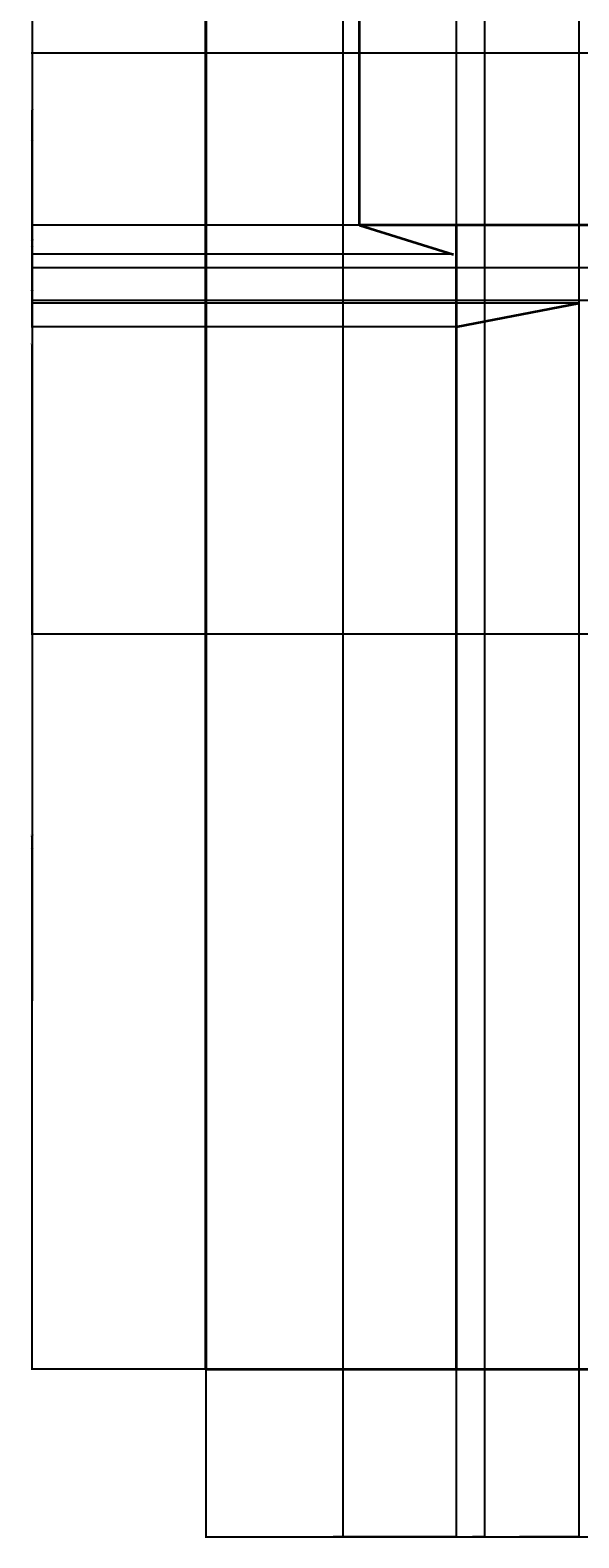
# Model space of a CAD drawing. Units: feet. Extents: x 4092 to 5585, y 725 to 1390.
# Tile 2 of 7: x 4921 to 5022, y 725 to 1001. Entities that reach past the tile are written whole.
import ezdxf

# ---------------------------------------------------------------- set-up
doc = ezdxf.new("R2010")
doc.units = ezdxf.units.FT
doc.layers.add('A-ANNO-DIMS', color=2, linetype='Continuous', lineweight=18)
doc.layers.add('A-ELEV', color=7, linetype='Continuous', lineweight=35)
doc.styles.get("Standard").update_dxf_attribs({"font": 'arial.ttf'})
doc.dimstyles.get("Standard").update_dxf_attribs({"dimtxt": 0.18, "dimasz": 0.18, "dimexe": 0.18, "dimexo": 0.0625, "dimgap": 0.09, "dimtad": 0, "dimtih": 1, "dimtoh": 1, "dimdec": 1, "dimzin": 0, "dimdsep": 46, "dimlunit": 3, "dimtxsty": 'Standard', "dimcen": 0.09, "dimadec": 0, "dimazin": 0, "dimtfac": 1, "dimtdec": 1, "dimtofl": 0, "dimtmove": 0, "dimatfit": 3, "dimfxl": 1, "dimtolj": 1, "dimtzin": 0, "dimarcsym": 0})

# ---------------------------------------------------------------- blocks, each defined once
blk = doc.blocks.new('*D4')
at = {"layer": 'A-ANNO-DIMS', "color": 0, "lineweight": -2, "transparency": 16777216}
for p, q in [((4953.29, 755.89), (4953.29, 725.07)), ((5553.29, 755.89), (5553.29, 725.07)), ((4953.47, 725.25), (5253, 725.25)), ((5553.11, 725.25), (5253.58, 725.25))]:
    blk.add_line(p, q, dxfattribs=at)
at = {"layer": 'A-ANNO-DIMS', "color": 0, "transparency": 16777216}
for points in [[(4953.47, 725.28), (4953.47, 725.22), (4953.29, 725.25)], [(5553.11, 725.28), (5553.11, 725.22), (5553.29, 725.25)]]:
    blk.add_solid(points, dxfattribs=at)
at = {"layer": 'Defpoints', "color": 0, "transparency": 16777216}
for p in [(4953.29, 755.95), (5553.29, 755.95), (5553.29, 725.25)]:
    blk.add_point(p, dxfattribs=at)
at = {"layer": 'A-ANNO-DIMS', "color": 0, "transparency": 16777216, "insert": (5253.29, 725.25), "char_height": 0.18, "attachment_point": 5}
blk.add_mtext('\\A1;600', dxfattribs=at)
blk = doc.blocks.new('*D17')
at = {"layer": 'A-ANNO-DIMS', "color": 0, "lineweight": -2, "transparency": 16777216}
for p, q in [((5021.54, 951.2), (4921.27, 951.2)), ((4921.45, 951.02), (4921.45, 853.76)), ((4921.45, 756.13), (4921.45, 853.39)), ((5285.73, 755.95), (4921.27, 755.95))]:
    blk.add_line(p, q, dxfattribs=at)
at = {"layer": 'A-ANNO-DIMS', "color": 0, "transparency": 16777216}
for points in [[(4921.42, 951.02), (4921.48, 951.02), (4921.45, 951.2)], [(4921.42, 756.13), (4921.48, 756.13), (4921.45, 755.95)]]:
    blk.add_solid(points, dxfattribs=at)
at = {"layer": 'Defpoints', "color": 0, "transparency": 16777216}
for p in [(4921.45, 951.2), (5021.61, 951.2), (5285.79, 755.95)]:
    blk.add_point(p, dxfattribs=at)
at = {"layer": 'A-ANNO-DIMS', "color": 0, "transparency": 16777216, "insert": (4921.45, 853.58), "char_height": 0.18, "attachment_point": 5}
blk.add_mtext('\\A1;195.25', dxfattribs=at)
blk = doc.blocks.new('*D18')
at = {"layer": 'A-ANNO-DIMS', "color": 0, "lineweight": -2, "transparency": 16777216}
for p, q in [((4978.29, 1010.79), (4921.27, 1010.79)), ((4921.45, 1010.61), (4921.45, 981.18)), ((4921.45, 951.38), (4921.45, 980.81)), ((5021.54, 951.2), (4921.27, 951.2))]:
    blk.add_line(p, q, dxfattribs=at)
at = {"layer": 'A-ANNO-DIMS', "color": 0, "transparency": 16777216}
for points in [[(4921.42, 1010.61), (4921.48, 1010.61), (4921.45, 1010.79)], [(4921.42, 951.38), (4921.48, 951.38), (4921.45, 951.2)]]:
    blk.add_solid(points, dxfattribs=at)
at = {"layer": 'Defpoints', "color": 0, "transparency": 16777216}
for p in [(4921.45, 1010.79), (4978.36, 1010.79), (5021.61, 951.2)]:
    blk.add_point(p, dxfattribs=at)
at = {"layer": 'A-ANNO-DIMS', "color": 0, "transparency": 16777216, "insert": (4921.45, 981), "char_height": 0.18, "attachment_point": 5}
blk.add_mtext('\\A1;59.59', dxfattribs=at)
blk = doc.blocks.new('*D24')
at = {"layer": 'A-ANNO-DIMS', "color": 0, "lineweight": -2, "transparency": 16777216}
for p, q in [((4953.29, 755.89), (4953.29, 725.07)), ((4999.11, 755.89), (4999.11, 725.07)), ((4953.47, 725.25), (4975.81, 725.25)), ((4998.93, 725.25), (4976.6, 725.25))]:
    blk.add_line(p, q, dxfattribs=at)
at = {"layer": 'A-ANNO-DIMS', "color": 0, "transparency": 16777216}
for points in [[(4953.47, 725.28), (4953.47, 725.22), (4953.29, 725.25)], [(4998.93, 725.28), (4998.93, 725.22), (4999.11, 725.25)]]:
    blk.add_solid(points, dxfattribs=at)
at = {"layer": 'Defpoints', "color": 0, "transparency": 16777216}
for p in [(4953.29, 755.95), (4999.11, 755.95), (4999.11, 725.25)]:
    blk.add_point(p, dxfattribs=at)
at = {"layer": 'A-ANNO-DIMS', "color": 0, "transparency": 16777216, "insert": (4976.2, 725.25), "char_height": 0.18, "attachment_point": 5}
blk.add_mtext('\\A1;45.82', dxfattribs=at)
blk = doc.blocks.new('*D25')
at = {"layer": 'A-ANNO-DIMS', "color": 0, "lineweight": -2, "transparency": 16777216}
for p, q in [((4999.11, 755.89), (4999.11, 725.07)), ((5021.61, 755.89), (5021.61, 725.07)), ((4999.29, 725.25), (5009.96, 725.25)), ((5021.43, 725.25), (5010.76, 725.25))]:
    blk.add_line(p, q, dxfattribs=at)
at = {"layer": 'A-ANNO-DIMS', "color": 0, "transparency": 16777216}
for points in [[(4999.29, 725.28), (4999.29, 725.22), (4999.11, 725.25)], [(5021.43, 725.28), (5021.43, 725.22), (5021.61, 725.25)]]:
    blk.add_solid(points, dxfattribs=at)
at = {"layer": 'Defpoints', "color": 0, "transparency": 16777216}
for p in [(4999.11, 755.95), (5021.61, 755.95), (5021.61, 725.25)]:
    blk.add_point(p, dxfattribs=at)
at = {"layer": 'A-ANNO-DIMS', "color": 0, "transparency": 16777216, "insert": (5010.36, 725.25), "char_height": 0.18, "attachment_point": 5}
blk.add_mtext('\\A1;22.49', dxfattribs=at)
blk = doc.blocks.new('*D26')
at = {"layer": 'A-ANNO-DIMS', "color": 0, "lineweight": -2, "transparency": 16777216}
for p, q in [((5021.61, 755.89), (5021.61, 725.07)), ((5028.8, 755.89), (5028.8, 725.07)), ((5021.79, 725.25), (5024.81, 725.25)), ((5028.62, 725.25), (5025.6, 725.25))]:
    blk.add_line(p, q, dxfattribs=at)
at = {"layer": 'A-ANNO-DIMS', "color": 0, "transparency": 16777216}
for points in [[(5021.79, 725.28), (5021.79, 725.22), (5021.61, 725.25)], [(5028.62, 725.28), (5028.62, 725.22), (5028.8, 725.25)]]:
    blk.add_solid(points, dxfattribs=at)
at = {"layer": 'Defpoints', "color": 0, "transparency": 16777216}
for p in [(5021.61, 755.95), (5028.8, 755.95), (5028.8, 725.25)]:
    blk.add_point(p, dxfattribs=at)
at = {"layer": 'A-ANNO-DIMS', "color": 0, "transparency": 16777216, "insert": (5025.2, 725.25), "char_height": 0.18, "attachment_point": 5}
blk.add_mtext('\\A1;7.194', dxfattribs=at)
blk = doc.blocks.new('*D43')
at = {"layer": 'A-ANNO-DIMS', "color": 0, "lineweight": -2, "transparency": 16777216}
for p, q in [((4999.05, 946.86), (4921.27, 946.86)), ((4921.45, 946.68), (4921.45, 851.59)), ((4921.45, 756.13), (4921.45, 851.22)), ((4953.23, 755.95), (4921.27, 755.95))]:
    blk.add_line(p, q, dxfattribs=at)
at = {"layer": 'A-ANNO-DIMS', "color": 0, "transparency": 16777216}
for points in [[(4921.42, 946.68), (4921.48, 946.68), (4921.45, 946.86)], [(4921.42, 756.13), (4921.48, 756.13), (4921.45, 755.95)]]:
    blk.add_solid(points, dxfattribs=at)
at = {"layer": 'Defpoints', "color": 0, "transparency": 16777216}
for p in [(4921.45, 946.86), (4999.11, 946.86), (4953.29, 755.95)]:
    blk.add_point(p, dxfattribs=at)
at = {"layer": 'A-ANNO-DIMS', "color": 0, "transparency": 16777216, "insert": (4921.45, 851.4), "char_height": 0.18, "attachment_point": 5}
blk.add_mtext('\\A1;190.9', dxfattribs=at)
blk = doc.blocks.new('*D44')
at = {"layer": 'A-ANNO-DIMS', "color": 0, "lineweight": -2, "transparency": 16777216}
for p, q in [((4998.6, 960.13), (4921.27, 960.13)), ((4921.45, 959.95), (4921.45, 953.68)), ((4921.45, 947.04), (4921.45, 953.31)), ((4999.05, 946.86), (4921.27, 946.86))]:
    blk.add_line(p, q, dxfattribs=at)
at = {"layer": 'A-ANNO-DIMS', "color": 0, "transparency": 16777216}
for points in [[(4921.42, 959.95), (4921.48, 959.95), (4921.45, 960.13)], [(4921.42, 947.04), (4921.48, 947.04), (4921.45, 946.86)]]:
    blk.add_solid(points, dxfattribs=at)
at = {"layer": 'Defpoints', "color": 0, "transparency": 16777216}
for p in [(4921.45, 960.13), (4998.66, 960.13), (4999.11, 946.86)]:
    blk.add_point(p, dxfattribs=at)
at = {"layer": 'A-ANNO-DIMS', "color": 0, "transparency": 16777216, "insert": (4921.45, 953.49), "char_height": 0.18, "attachment_point": 5}
blk.add_mtext('\\A1;13.268', dxfattribs=at)
blk = doc.blocks.new('*D45')
at = {"layer": 'A-ANNO-DIMS', "color": 0, "lineweight": -2, "transparency": 16777216}
for p, q in [((4981.38, 965.48), (4921.27, 965.48)), ((4921.45, 965.3), (4921.45, 962.99)), ((4921.45, 960.31), (4921.45, 962.62)), ((4998.6, 960.13), (4921.27, 960.13))]:
    blk.add_line(p, q, dxfattribs=at)
at = {"layer": 'A-ANNO-DIMS', "color": 0, "transparency": 16777216}
for points in [[(4921.42, 965.3), (4921.48, 965.3), (4921.45, 965.48)], [(4921.42, 960.31), (4921.48, 960.31), (4921.45, 960.13)]]:
    blk.add_solid(points, dxfattribs=at)
at = {"layer": 'Defpoints', "color": 0, "transparency": 16777216}
for p in [(4921.45, 965.48), (4981.44, 965.48), (4998.66, 960.13)]:
    blk.add_point(p, dxfattribs=at)
at = {"layer": 'A-ANNO-DIMS', "color": 0, "transparency": 16777216, "insert": (4921.45, 962.8), "char_height": 0.18, "attachment_point": 5}
blk.add_mtext('\\A1;5.351', dxfattribs=at)
blk = doc.blocks.new('*D46')
at = {"layer": 'A-ANNO-DIMS', "color": 0, "lineweight": -2, "transparency": 16777216}
for p, q in [((4978.29, 1007.95), (4921.27, 1007.95)), ((4921.45, 1007.77), (4921.45, 986.89)), ((4921.45, 965.66), (4921.45, 986.53)), ((4981.38, 965.48), (4921.27, 965.48))]:
    blk.add_line(p, q, dxfattribs=at)
at = {"layer": 'A-ANNO-DIMS', "color": 0, "transparency": 16777216}
for points in [[(4921.42, 1007.77), (4921.48, 1007.77), (4921.45, 1007.95)], [(4921.42, 965.66), (4921.48, 965.66), (4921.45, 965.48)]]:
    blk.add_solid(points, dxfattribs=at)
at = {"layer": 'Defpoints', "color": 0, "transparency": 16777216}
for p in [(4921.45, 1007.95), (4978.36, 1007.95), (4981.44, 965.48)]:
    blk.add_point(p, dxfattribs=at)
at = {"layer": 'A-ANNO-DIMS', "color": 0, "transparency": 16777216, "insert": (4921.45, 986.71), "char_height": 0.18, "attachment_point": 5}
blk.add_mtext('\\A1;42.47', dxfattribs=at)
blk = doc.blocks.new('*D47')
at = {"layer": 'A-ANNO-DIMS', "color": 0, "lineweight": -2, "transparency": 16777216}
for p, q in [((4978.36, 1010.73), (4978.36, 725.07)), ((4999.11, 1010.73), (4999.11, 725.07)), ((4978.54, 725.25), (4988.34, 725.25)), ((4998.93, 725.25), (4989.13, 725.25))]:
    blk.add_line(p, q, dxfattribs=at)
at = {"layer": 'A-ANNO-DIMS', "color": 0, "transparency": 16777216}
for points in [[(4978.54, 725.28), (4978.54, 725.22), (4978.36, 725.25)], [(4998.93, 725.28), (4998.93, 725.22), (4999.11, 725.25)]]:
    blk.add_solid(points, dxfattribs=at)
at = {"layer": 'Defpoints', "color": 0, "transparency": 16777216}
for p in [(4978.36, 1010.79), (4999.11, 1010.79), (4999.11, 725.25)]:
    blk.add_point(p, dxfattribs=at)
at = {"layer": 'A-ANNO-DIMS', "color": 0, "transparency": 16777216, "insert": (4988.74, 725.25), "char_height": 0.18, "attachment_point": 5}
blk.add_mtext('\\A1;20.76', dxfattribs=at)
blk = doc.blocks.new('*D48')
at = {"layer": 'A-ANNO-DIMS', "color": 0, "lineweight": -2, "transparency": 16777216}
for p, q in [((4999.11, 1010.73), (4999.11, 725.07)), ((5004.32, 1010.73), (5004.32, 725.07)), ((4999.29, 725.25), (5001.32, 725.25)), ((5004.14, 725.25), (5002.11, 725.25))]:
    blk.add_line(p, q, dxfattribs=at)
at = {"layer": 'A-ANNO-DIMS', "color": 0, "transparency": 16777216}
for points in [[(4999.29, 725.28), (4999.29, 725.22), (4999.11, 725.25)], [(5004.14, 725.28), (5004.14, 725.22), (5004.32, 725.25)]]:
    blk.add_solid(points, dxfattribs=at)
at = {"layer": 'Defpoints', "color": 0, "transparency": 16777216}
for p in [(4999.11, 1010.79), (5004.32, 1010.79), (5004.32, 725.25)]:
    blk.add_point(p, dxfattribs=at)
at = {"layer": 'A-ANNO-DIMS', "color": 0, "transparency": 16777216, "insert": (5001.72, 725.25), "char_height": 0.18, "attachment_point": 5}
blk.add_mtext('\\A1;5.203', dxfattribs=at)
blk = doc.blocks.new('*D49')
at = {"layer": 'A-ANNO-DIMS', "color": 0, "lineweight": -2, "transparency": 16777216}
for p, q in [((5004.32, 1010.73), (5004.32, 725.07)), ((5021.61, 1010.73), (5021.61, 725.07)), ((5004.5, 725.25), (5012.58, 725.25)), ((5021.43, 725.25), (5013.35, 725.25))]:
    blk.add_line(p, q, dxfattribs=at)
at = {"layer": 'A-ANNO-DIMS', "color": 0, "transparency": 16777216}
for points in [[(5004.5, 725.28), (5004.5, 725.22), (5004.32, 725.25)], [(5021.43, 725.28), (5021.43, 725.22), (5021.61, 725.25)]]:
    blk.add_solid(points, dxfattribs=at)
at = {"layer": 'Defpoints', "color": 0, "transparency": 16777216}
for p in [(5004.32, 1010.79), (5021.61, 1010.79), (5021.61, 725.25)]:
    blk.add_point(p, dxfattribs=at)
at = {"layer": 'A-ANNO-DIMS', "color": 0, "transparency": 16777216, "insert": (5012.96, 725.25), "char_height": 0.18, "attachment_point": 5}
blk.add_mtext('\\A1;17.29', dxfattribs=at)
blk = doc.blocks.new('*D50')
at = {"layer": 'A-ANNO-DIMS', "color": 0, "lineweight": -2, "transparency": 16777216}
for p, q in [((5021.61, 1010.73), (5021.61, 725.07)), ((5028.8, 1010.73), (5028.8, 725.07)), ((5021.79, 725.25), (5024.81, 725.25)), ((5028.62, 725.25), (5025.6, 725.25))]:
    blk.add_line(p, q, dxfattribs=at)
at = {"layer": 'A-ANNO-DIMS', "color": 0, "transparency": 16777216}
for points in [[(5021.79, 725.28), (5021.79, 725.22), (5021.61, 725.25)], [(5028.62, 725.28), (5028.62, 725.22), (5028.8, 725.25)]]:
    blk.add_solid(points, dxfattribs=at)
at = {"layer": 'Defpoints', "color": 0, "transparency": 16777216}
for p in [(5021.61, 1010.79), (5028.8, 1010.79), (5028.8, 725.25)]:
    blk.add_point(p, dxfattribs=at)
at = {"layer": 'A-ANNO-DIMS', "color": 0, "transparency": 16777216, "insert": (5025.2, 725.25), "char_height": 0.18, "attachment_point": 5}
blk.add_mtext('\\A1;7.194', dxfattribs=at)
blk = doc.blocks.new('*D71')
at = {"layer": 'A-ANNO-DIMS', "color": 0, "lineweight": -2, "transparency": 16777216}
for p, q in [((5285.73, 890.54), (4921.27, 890.54)), ((4921.45, 890.36), (4921.45, 823.43)), ((4921.45, 756.13), (4921.45, 823.06)), ((5285.73, 755.95), (4921.27, 755.95))]:
    blk.add_line(p, q, dxfattribs=at)
at = {"layer": 'A-ANNO-DIMS', "color": 0, "transparency": 16777216}
for points in [[(4921.42, 890.36), (4921.48, 890.36), (4921.45, 890.54)], [(4921.42, 756.13), (4921.48, 756.13), (4921.45, 755.95)]]:
    blk.add_solid(points, dxfattribs=at)
at = {"layer": 'Defpoints', "color": 0, "transparency": 16777216}
for p in [(4921.45, 890.54), (5285.79, 890.54), (5285.79, 755.95)]:
    blk.add_point(p, dxfattribs=at)
at = {"layer": 'A-ANNO-DIMS', "color": 0, "transparency": 16777216, "insert": (4921.45, 823.24), "char_height": 0.18, "attachment_point": 5}
blk.add_mtext('\\A1;134.6', dxfattribs=at)
blk = doc.blocks.new('*D72')
at = {"layer": 'A-ANNO-DIMS', "color": 0, "lineweight": -2, "transparency": 16777216}
for p, q in [((5285.73, 996.97), (4921.27, 996.97)), ((4921.45, 996.79), (4921.45, 943.94)), ((4921.45, 890.72), (4921.45, 943.57)), ((5285.73, 890.54), (4921.27, 890.54))]:
    blk.add_line(p, q, dxfattribs=at)
at = {"layer": 'A-ANNO-DIMS', "color": 0, "transparency": 16777216}
for points in [[(4921.42, 996.79), (4921.48, 996.79), (4921.45, 996.97)], [(4921.42, 890.72), (4921.48, 890.72), (4921.45, 890.54)]]:
    blk.add_solid(points, dxfattribs=at)
at = {"layer": 'Defpoints', "color": 0, "transparency": 16777216}
for p in [(4921.45, 996.97), (5285.79, 996.97), (5285.79, 890.54)]:
    blk.add_point(p, dxfattribs=at)
at = {"layer": 'A-ANNO-DIMS', "color": 0, "transparency": 16777216, "insert": (4921.45, 943.75), "char_height": 0.18, "attachment_point": 5}
blk.add_mtext('\\A1;106.43', dxfattribs=at)
blk = doc.blocks.new('*D75')
at = {"layer": 'A-ANNO-DIMS', "color": 0, "lineweight": -2, "transparency": 16777216}
for p, q in [((5392.49, 951.65), (4921.27, 951.65)), ((4921.45, 951.47), (4921.45, 853.98)), ((4921.45, 756.13), (4921.45, 853.62)), ((5392.49, 755.95), (4921.27, 755.95))]:
    blk.add_line(p, q, dxfattribs=at)
at = {"layer": 'A-ANNO-DIMS', "color": 0, "transparency": 16777216}
for points in [[(4921.42, 951.47), (4921.48, 951.47), (4921.45, 951.65)], [(4921.42, 756.13), (4921.48, 756.13), (4921.45, 755.95)]]:
    blk.add_solid(points, dxfattribs=at)
at = {"layer": 'Defpoints', "color": 0, "transparency": 16777216}
for p in [(4921.45, 951.65), (5392.55, 951.65), (5392.55, 755.95)]:
    blk.add_point(p, dxfattribs=at)
at = {"layer": 'A-ANNO-DIMS', "color": 0, "transparency": 16777216, "insert": (4921.45, 853.8), "char_height": 0.18, "attachment_point": 5}
blk.add_mtext('\\A1;195.7', dxfattribs=at)
blk = doc.blocks.new('*D76')
at = {"layer": 'A-ANNO-DIMS', "color": 0, "lineweight": -2, "transparency": 16777216}
for p, q in [((5392.49, 957.65), (4921.27, 957.65)), ((4921.45, 957.47), (4921.45, 954.83)), ((4921.45, 951.83), (4921.45, 954.46)), ((5392.49, 951.65), (4921.27, 951.65))]:
    blk.add_line(p, q, dxfattribs=at)
at = {"layer": 'A-ANNO-DIMS', "color": 0, "transparency": 16777216}
for points in [[(4921.42, 957.47), (4921.48, 957.47), (4921.45, 957.65)], [(4921.42, 951.83), (4921.48, 951.83), (4921.45, 951.65)]]:
    blk.add_solid(points, dxfattribs=at)
at = {"layer": 'Defpoints', "color": 0, "transparency": 16777216}
for p in [(4921.45, 957.65), (5392.55, 957.65), (5392.55, 951.65)]:
    blk.add_point(p, dxfattribs=at)
at = {"layer": 'A-ANNO-DIMS', "color": 0, "transparency": 16777216, "insert": (4921.45, 954.65), "char_height": 0.18, "attachment_point": 5}
blk.add_mtext('\\A1;6', dxfattribs=at)
blk = doc.blocks.new('*D77')
at = {"layer": 'A-ANNO-DIMS', "color": 0, "lineweight": -2, "transparency": 16777216}
for p, q in [((5392.49, 965.48), (4921.27, 965.48)), ((4921.45, 965.3), (4921.45, 961.74)), ((4921.45, 957.83), (4921.45, 961.38)), ((5392.49, 957.65), (4921.27, 957.65))]:
    blk.add_line(p, q, dxfattribs=at)
at = {"layer": 'A-ANNO-DIMS', "color": 0, "transparency": 16777216}
for points in [[(4921.42, 965.3), (4921.48, 965.3), (4921.45, 965.48)], [(4921.42, 957.83), (4921.48, 957.83), (4921.45, 957.65)]]:
    blk.add_solid(points, dxfattribs=at)
at = {"layer": 'Defpoints', "color": 0, "transparency": 16777216}
for p in [(4921.45, 965.48), (5392.55, 965.48), (5392.55, 957.65)]:
    blk.add_point(p, dxfattribs=at)
at = {"layer": 'A-ANNO-DIMS', "color": 0, "transparency": 16777216, "insert": (4921.45, 961.56), "char_height": 0.18, "attachment_point": 5}
blk.add_mtext('\\A1;7.833', dxfattribs=at)
blk = doc.blocks.new('*D78')
at = {"layer": 'A-ANNO-DIMS', "color": 0, "lineweight": -2, "transparency": 16777216}
for p, q in [((5392.49, 1007.95), (4921.27, 1007.95)), ((4921.45, 1007.77), (4921.45, 986.89)), ((4921.45, 965.66), (4921.45, 986.53)), ((5392.49, 965.48), (4921.27, 965.48))]:
    blk.add_line(p, q, dxfattribs=at)
at = {"layer": 'A-ANNO-DIMS', "color": 0, "transparency": 16777216}
for points in [[(4921.42, 1007.77), (4921.48, 1007.77), (4921.45, 1007.95)], [(4921.42, 965.66), (4921.48, 965.66), (4921.45, 965.48)]]:
    blk.add_solid(points, dxfattribs=at)
at = {"layer": 'Defpoints', "color": 0, "transparency": 16777216}
for p in [(4921.45, 1007.95), (5392.55, 1007.95), (5392.55, 965.48)]:
    blk.add_point(p, dxfattribs=at)
at = {"layer": 'A-ANNO-DIMS', "color": 0, "transparency": 16777216, "insert": (4921.45, 986.71), "char_height": 0.18, "attachment_point": 5}
blk.add_mtext('\\A1;42.47', dxfattribs=at)

msp = doc.modelspace()

# ---------------------------------------------------------------- linework, layer by layer
at = {"layer": 'A-ELEV'}
for p, q in [((4953.293, 755.9488), (4953.293, 1253.9488)), ((4981.4448, 965.4789), (4998.659, 960.128)), ((4999.1145, 946.8601), (5021.6062, 951.2024)), ((4953.293, 755.9488), (5553.293, 755.9488))]:
    msp.add_line(p, q, dxfattribs=at)
for points in [[(4953.293, 755.9488), (5231.15, 755.9488), (5231.15, 1253.9488), (4953.293, 1253.9488)], [(4981.4448, 1007.9488), (5202.5428, 1007.9488), (5202.5428, 965.4789), (4981.4448, 965.4789)]]:
    msp.add_lwpolyline(points, close=True, dxfattribs=at)
msp.add_lwpolyline([(4999.1145, 965.4789), (4999.1145, 755.9488)], dxfattribs=at)

# ---------------------------------------------------------------- dimensions: what is measured, and where the dimension line sits
at = {"layer": 'A-ANNO-DIMS'}
for base, p1, p2, override, picture, middle in [((4921.4517, 1010.7906), (5021.6062, 951.2024), (4978.3561, 1010.7906), {"dimdec": 2, "dimlfac": 1, "dimrnd": 0, "dimzin": 0, "dimdsep": 46, "dimlunit": 2}, '*D18', (4921.4517, 980.9965)), ((4921.4517, 1007.9488), (4981.4448, 965.4789), (4978.3561, 1007.9488), {"dimdec": 2, "dimlfac": 1, "dimrnd": 0, "dimzin": 0, "dimdsep": 46, "dimlunit": 2}, '*D46', (4921.4517, 986.7139)), ((4921.4517, 1007.9488), (5392.5521, 965.4789), (5392.5521, 1007.9488), {"dimdec": 2, "dimlfac": 1, "dimrnd": 0, "dimzin": 0, "dimdsep": 46, "dimlunit": 2}, '*D78', (4921.4517, 986.7139)), ((4921.4517, 996.9712), (5285.7915, 890.5384), (5285.7915, 996.9712), {"dimdec": 2, "dimlfac": 1, "dimrnd": 0, "dimzin": 0, "dimdsep": 46, "dimlunit": 2}, '*D72', (4921.4517, 943.7548)), ((4921.4517, 965.4789), (4998.659, 960.128), (4981.4448, 965.4789), {"dimdec": 3, "dimlfac": 1, "dimrnd": 0, "dimzin": 0, "dimdsep": 46, "dimlunit": 2}, '*D45', (4921.4517, 962.8035)), ((4921.4517, 965.4789), (5392.5521, 957.6463), (5392.5521, 965.4789), {"dimdec": 3, "dimlfac": 1, "dimrnd": 0, "dimzin": 0, "dimdsep": 46, "dimlunit": 2}, '*D77', (4921.4517, 961.5626)), ((4921.4517, 960.128), (4999.1145, 946.8601), (4998.659, 960.128), {"dimdec": 3, "dimlfac": 1, "dimrnd": 0, "dimzin": 0, "dimdsep": 46, "dimlunit": 2}, '*D44', (4921.4517, 953.4941)), ((4921.4517, 957.6463), (5392.5521, 951.6463), (5392.5521, 957.6463), {"dimdec": 0, "dimlfac": 1, "dimrnd": 0, "dimzin": 0, "dimdsep": 46, "dimlunit": 2}, '*D76', (4921.4517, 954.6463)), ((4921.4517, 951.2024), (5285.7915, 755.9488), (5021.6062, 951.2024), {"dimdec": 2, "dimlfac": 1, "dimrnd": 0, "dimzin": 0, "dimdsep": 46, "dimlunit": 2}, '*D17', (4921.4517, 853.5756)), ((4921.4517, 951.6463), (5392.5521, 755.9488), (5392.5521, 951.6463), {"dimdec": 1, "dimlfac": 1, "dimrnd": 0, "dimzin": 0, "dimdsep": 46, "dimlunit": 2}, '*D75', (4921.4517, 853.7975)), ((4921.4517, 946.8601), (4953.293, 755.9488), (4999.1145, 946.8601), {"dimdec": 1, "dimlfac": 1, "dimrnd": 0, "dimzin": 0, "dimdsep": 46, "dimlunit": 2}, '*D43', (4921.4517, 851.4044)), ((4921.4517, 890.5384), (5285.7915, 755.9488), (5285.7915, 890.5384), {"dimdec": 1, "dimlfac": 1, "dimrnd": 0, "dimzin": 0, "dimdsep": 46, "dimlunit": 2}, '*D71', (4921.4517, 823.2436))]:
    dim = msp.add_linear_dim(base=base, p1=p1, p2=p2, angle=90, dimstyle='Standard', override=override, dxfattribs=at)
    dim.commit()
    dim.dimension.update_dxf_attribs({"geometry": picture, "text_midpoint": middle})
for base, p1, p2, override, picture, middle in [((4999.1145, 725.2488), (4978.3561, 1010.7906), (4999.1145, 1010.7906), {"dimdec": 2, "dimlfac": 1, "dimrnd": 0, "dimzin": 0, "dimdsep": 46, "dimlunit": 2}, '*D47', (4988.7353, 725.2488)), ((5004.3171, 725.2488), (4999.1145, 1010.7906), (5004.3171, 1010.7906), {"dimdec": 3, "dimlfac": 1, "dimrnd": 0, "dimzin": 0, "dimdsep": 46, "dimlunit": 2}, '*D48', (5001.7158, 725.2488)), ((5021.6062, 725.2488), (5004.3171, 1010.7906), (5021.6062, 1010.7906), {"dimdec": 2, "dimlfac": 1, "dimrnd": 0, "dimzin": 0, "dimdsep": 46, "dimlunit": 2}, '*D49', (5012.9616, 725.2488)), ((5028.8002, 725.2488), (5021.6062, 1010.7906), (5028.8002, 1010.7906), {"dimdec": 3, "dimlfac": 1, "dimrnd": 0, "dimzin": 0, "dimdsep": 46, "dimlunit": 2}, '*D50', (5025.2032, 725.2488)), ((5553.293, 725.2488), (4953.293, 755.9488), (5553.293, 755.9488), {"dimdec": 0, "dimlfac": 1, "dimrnd": 0, "dimzin": 0, "dimdsep": 46, "dimlunit": 2}, '*D4', (5253.293, 725.2488)), ((4999.1145, 725.2488), (4953.293, 755.9488), (4999.1145, 755.9488), {"dimdec": 2, "dimlfac": 1, "dimrnd": 0, "dimzin": 0, "dimdsep": 46, "dimlunit": 2}, '*D24', (4976.2037, 725.2488)), ((5021.6062, 725.2488), (4999.1145, 755.9488), (5021.6062, 755.9488), {"dimdec": 2, "dimlfac": 1, "dimrnd": 0, "dimzin": 0, "dimdsep": 46, "dimlunit": 2}, '*D25', (5010.3603, 725.2488)), ((5028.8002, 725.2488), (5021.6062, 755.9488), (5028.8002, 755.9488), {"dimdec": 3, "dimlfac": 1, "dimrnd": 0, "dimzin": 0, "dimdsep": 46, "dimlunit": 2}, '*D26', (5025.2032, 725.2488))]:
    dim = msp.add_linear_dim(base=base, p1=p1, p2=p2, dimstyle='Standard', override=override, dxfattribs=at)
    dim.commit()
    dim.dimension.update_dxf_attribs({"geometry": picture, "text_midpoint": middle})

doc.saveas('drawing.dxf')
